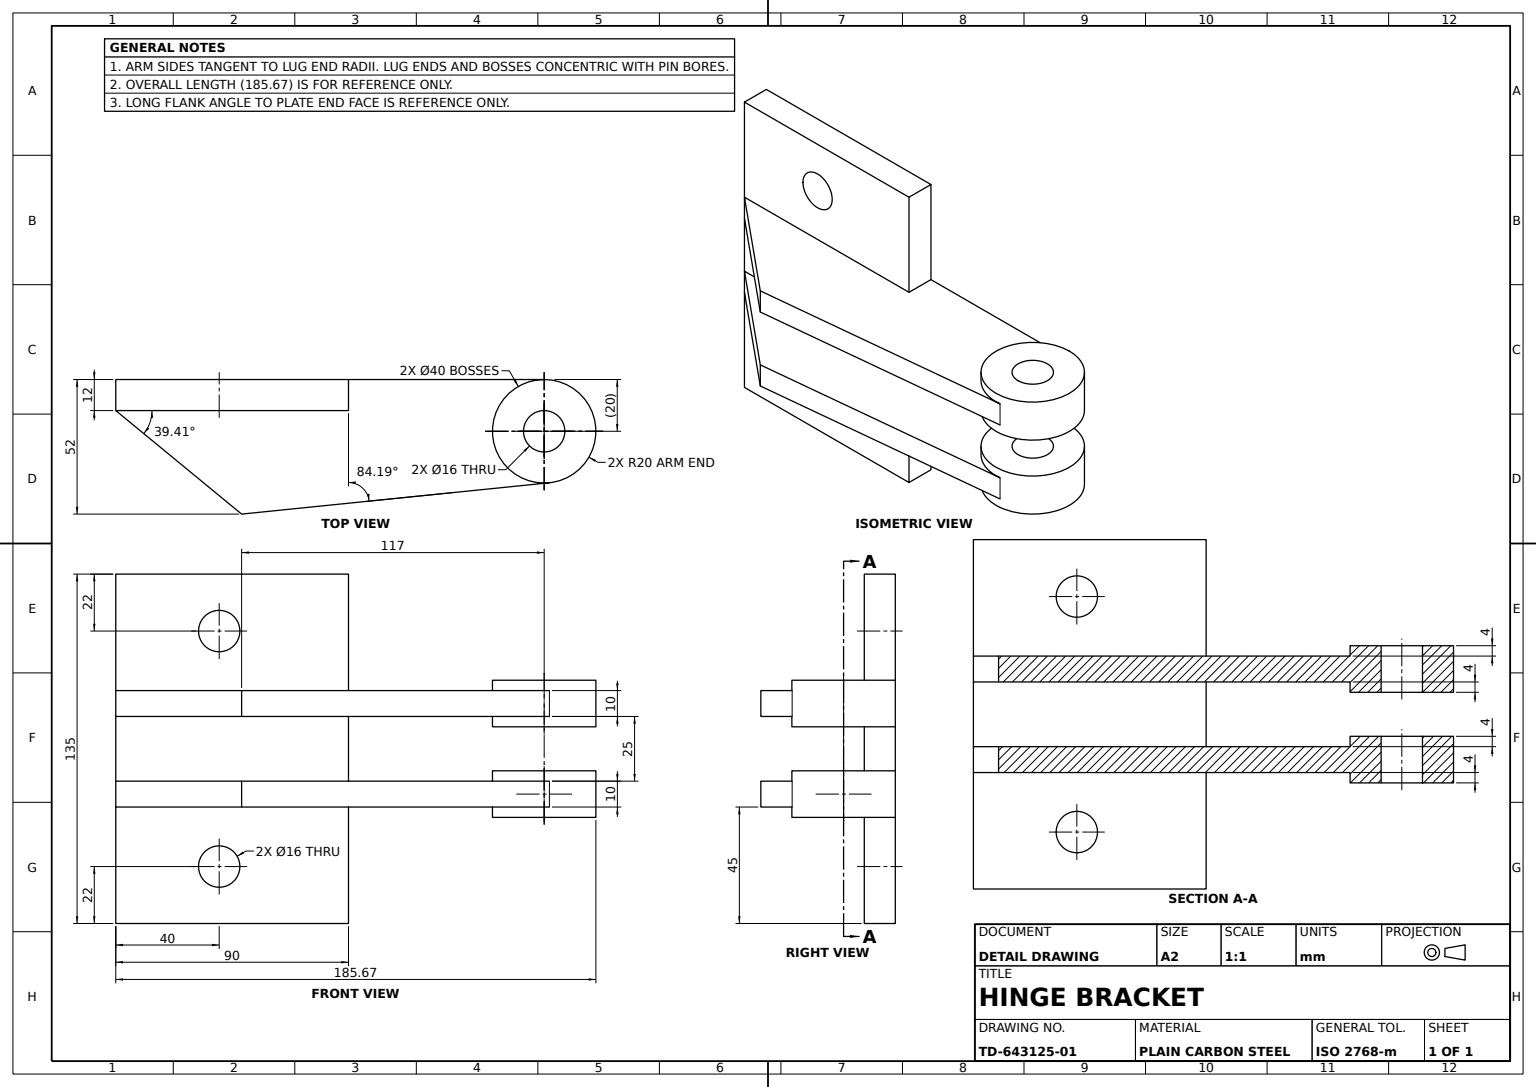
from build123d import *

# Parameters (mm, degrees)
BASE_PLATE_SKETCH_W        = 90
BASE_PLATE_SKETCH_H        = 135
BASE_PLATE_DEPTH           = 12
MOUNTING_HOLES_SKETCH_R    = 8
MOUNTING_HOLES_2X_16_DEPTH = 22
CLEVIS_ARM_SKETCH_R        = 20
CLEVIS_ARM_SKETCH_R_2      = 8
CLEVIS_ARM_DEPTH           = 22.5
CLEVIS_SLOT_DEPTH          = 162.074413963
CLEVIS_SLOT_DEPTH_BACK     = 162.074413963
CLEVIS_SLOT_SKETCH_W       = 40
CLEVIS_SLOT_SKETCH_H       = 25
PIN_HOLE_DEPTH             = 165.465701085
PIN_HOLE_DEPTH_BACK        = 165.465701085
PIN_HOLE_SKETCH_W          = 94.002676874
PIN_HOLE_SKETCH_H          = 25
LUG_BOSS_1_SKETCH_R        = 20
LUG_BOSS_1_SKETCH_R_2      = 8
LUG_BOSS_1_40_DEPTH        = 4
LUG_START                  = 4
LUG_BOSS_2_SKETCH_R        = 20
LUG_BOSS_2_SKETCH_R_2      = 8
LUG_BOSS_2_40_DEPTH        = 4
LUG_BOSS_3_SKETCH_R        = 20
LUG_BOSS_3_SKETCH_R_2      = 8
LUG_BOSS_3_40_DEPTH        = 4
LUG_BOSS_4_SKETCH_R        = 20
LUG_BOSS_4_SKETCH_R_2      = 8
LUG_BOSS_4_40_DEPTH        = 4


with BuildPart() as part:
    # Base Plate Sketch → Base Plate (new body)
    with BuildSketch(Plane.XY):
        Rectangle(BASE_PLATE_SKETCH_W, BASE_PLATE_SKETCH_H)
    extrude(amount=BASE_PLATE_DEPTH)

    # Mounting Holes Sketch → Mounting Holes 2xØ16 (cut)
    with BuildSketch(Plane.XY.offset(12)):
        with Locations((5, -45.5)):
            Circle(MOUNTING_HOLES_SKETCH_R)
        with Locations((5, 45.5)):
            Circle(MOUNTING_HOLES_SKETCH_R)
    extrude(amount=-MOUNTING_HOLES_2X_16_DEPTH, mode=Mode.SUBTRACT)

    # Clevis Arm Sketch → Clevis Arm (add, symmetric)
    # profile 1 of 2: a face of its own
    with BuildSketch(Plane(origin=(0, 0, 0), x_dir=(1, 0, 0), z_dir=(0, 1, 0))):
        with BuildLine():
            Line((-120.672374095, -12), (-45, -12))
            Line((-45, -12), (-45, 0))
            Line((-45, 0), (45, 0))
            Line((45, 0), (-3.672374095, 40))
            Line((-3.672374095, 40), (-122.695594955, 27.897401271))
            ThreePointArc((-122.695594955, 27.897401271), (-107.264622926, 22.84022266), (-100.672374095, 8))
            ThreePointArc((-100.672374095, 8), (-106.530238471, -6.142135624), (-120.672374095, -12))
        make_face()
    # profile 2 of 2: a face of its own
    with BuildSketch(Plane(origin=(0, 0, 0), x_dir=(1, 0, 0), z_dir=(0, 1, 0))):
        with Locations((-120.672374095, 8)):
            Circle(CLEVIS_ARM_SKETCH_R)
        with Locations(Location((-120.672374095, 8, 0), (0, 0, 90))):
            Circle(CLEVIS_ARM_SKETCH_R_2, mode=Mode.SUBTRACT)
    extrude(amount=CLEVIS_ARM_DEPTH, both=True)

    # Clevis Slot Sketch → Clevis Slot (cut, two sides: drawn at the far end of the back side and taken through both)
    with BuildSketch(Plane(origin=(0, 0, 0), x_dir=(0, 0, -1), z_dir=(1, 0, 0)).offset(-CLEVIS_SLOT_DEPTH_BACK)):
        with Locations((20, 0)):
            Rectangle(CLEVIS_SLOT_SKETCH_W, CLEVIS_SLOT_SKETCH_H)
    extrude(amount=CLEVIS_SLOT_DEPTH + CLEVIS_SLOT_DEPTH_BACK, mode=Mode.SUBTRACT)

    # Pin Hole Sketch → Pin Hole (cut, two sides: drawn at the far end of the back side and taken through both)
    with BuildSketch(Plane.XY.offset(12).offset(-PIN_HOLE_DEPTH_BACK)):
        with Locations((-92.001338437, 0)):
            Rectangle(PIN_HOLE_SKETCH_W, PIN_HOLE_SKETCH_H)
    extrude(amount=PIN_HOLE_DEPTH + PIN_HOLE_DEPTH_BACK, mode=Mode.SUBTRACT)

    # Lug Boss 1 Sketch → Lug Boss 1 Ø40 (add)
    with BuildSketch(Plane.XZ.offset(22.5)):
        with Locations(Location((-120.672374095, -8, 0), (0, 0, 270))):
            Circle(LUG_BOSS_1_SKETCH_R)
        with Locations(Location((-120.672374095, -8, 0), (0, 0, 270))):
            Circle(LUG_BOSS_1_SKETCH_R_2, mode=Mode.SUBTRACT)
    extrude(amount=LUG_BOSS_1_40_DEPTH)

    # Lug Boss 2 Sketch → Lug Boss 2 Ø40 (add)
    with BuildSketch(Plane(origin=(0, -12.5, 0), x_dir=(1, 0, 0), z_dir=(0, 1, 0)).offset(LUG_START)):
        with Locations(Location((-120.672374095, 8, 0), (0, 0, 90))):
            Circle(LUG_BOSS_2_SKETCH_R)
        with Locations(Location((-120.672374095, 8, 0), (0, 0, 90))):
            Circle(LUG_BOSS_2_SKETCH_R_2, mode=Mode.SUBTRACT)
    extrude(amount=-LUG_BOSS_2_40_DEPTH)

    # Lug Boss 3 Sketch → Lug Boss 3 Ø40 (add)
    with BuildSketch(Plane(origin=(0, 22.5, 0), x_dir=(1, 0, 0), z_dir=(0, 1, 0)).offset(LUG_START)):
        with Locations(Location((-120.672374095, 8, 0), (0, 0, 270))):
            Circle(LUG_BOSS_3_SKETCH_R)
        with Locations(Location((-120.672374095, 8, 0), (0, 0, 90))):
            Circle(LUG_BOSS_3_SKETCH_R_2, mode=Mode.SUBTRACT)
    extrude(amount=-LUG_BOSS_3_40_DEPTH)

    # Lug Boss 4 Sketch → Lug Boss 4 Ø40 (add)
    with BuildSketch(Plane.XZ.offset(-12.5)):
        with Locations(Location((-120.672374095, -8, 0), (0, 0, 270))):
            Circle(LUG_BOSS_4_SKETCH_R)
        with Locations(Location((-120.672374095, -8, 0), (0, 0, 270))):
            Circle(LUG_BOSS_4_SKETCH_R_2, mode=Mode.SUBTRACT)
    extrude(amount=LUG_BOSS_4_40_DEPTH)


solid = part.part
